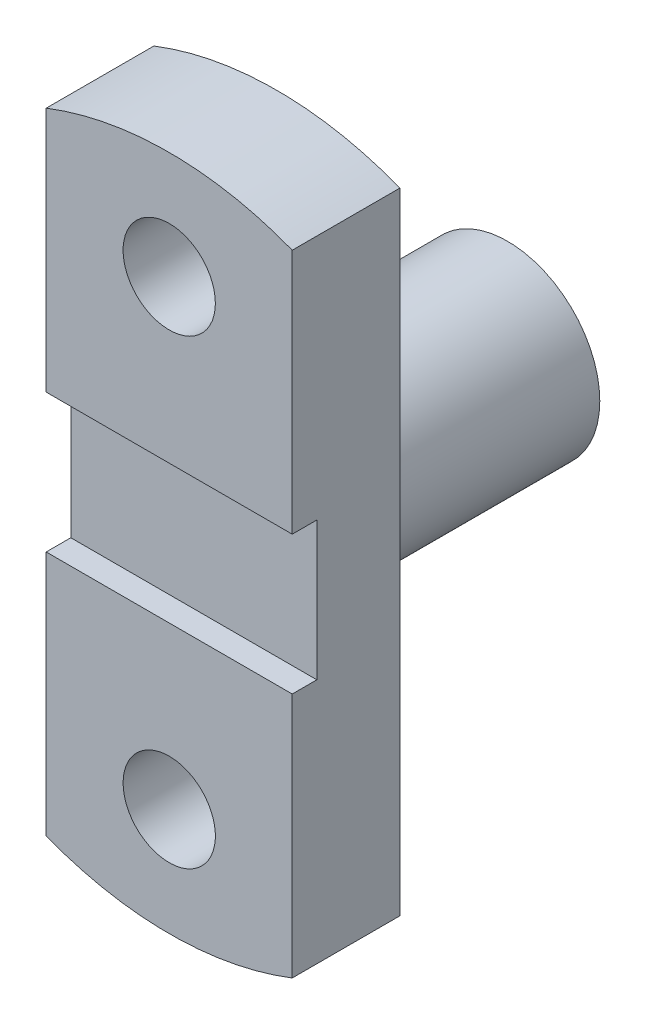
from build123d import *

# Parameters (mm, degrees)
PLATE_PROFILE_SKETCH_R    = 15
KEEPER_PLATE_BODY_DEPTH   = 17.5
MOUNTING_HOLES_SKETCH_W   = 8
MOUNTING_HOLES_SKETCH_H   = 45
MOUNTING_HOLES_DEPTH      = 80
BOSS_60_SKETCH_R          = 30
CYLINDRICAL_BOSS_60_DEPTH = 75


with BuildPart() as part:
    # Plate Profile Sketch → Keeper Plate Body (new, symmetric)
    with BuildSketch(Plane.XY):
        with BuildLine():
            Line((-40, -102.46950766), (-40, 102.46950766))
            ThreePointArc((-40, 102.46950766), (0, 110), (40, 102.46950766))
            Line((40, 102.46950766), (40, -102.46950766))
            ThreePointArc((40, -102.46950766), (0, -110), (-40, -102.46950766))
        make_face()
        with Locations((0, 75)):
            Circle(PLATE_PROFILE_SKETCH_R, mode=Mode.SUBTRACT)
        with Locations(Location((0, -75, 0), (0, 0, 180))):
            Circle(PLATE_PROFILE_SKETCH_R, mode=Mode.SUBTRACT)
    extrude(amount=KEEPER_PLATE_BODY_DEPTH, both=True)

    # Mounting Holes Sketch → Mounting Holes (cut)
    with BuildSketch(Plane(origin=(40, 0, 0), x_dir=(0, 0, -1), z_dir=(1, 0, 0))):
        with Locations((-13.5, 0)):
            Rectangle(MOUNTING_HOLES_SKETCH_W, MOUNTING_HOLES_SKETCH_H)
    extrude(amount=-MOUNTING_HOLES_DEPTH, mode=Mode.SUBTRACT)

    # Boss Ø60 Sketch → Cylindrical Boss Ø60 (add)
    with BuildSketch(Plane(origin=(0, 0, -17.5), x_dir=(-1, 0, 0), z_dir=(0, 0, -1))):
        Circle(BOSS_60_SKETCH_R)
    extrude(amount=CYLINDRICAL_BOSS_60_DEPTH)


solid = part.part
